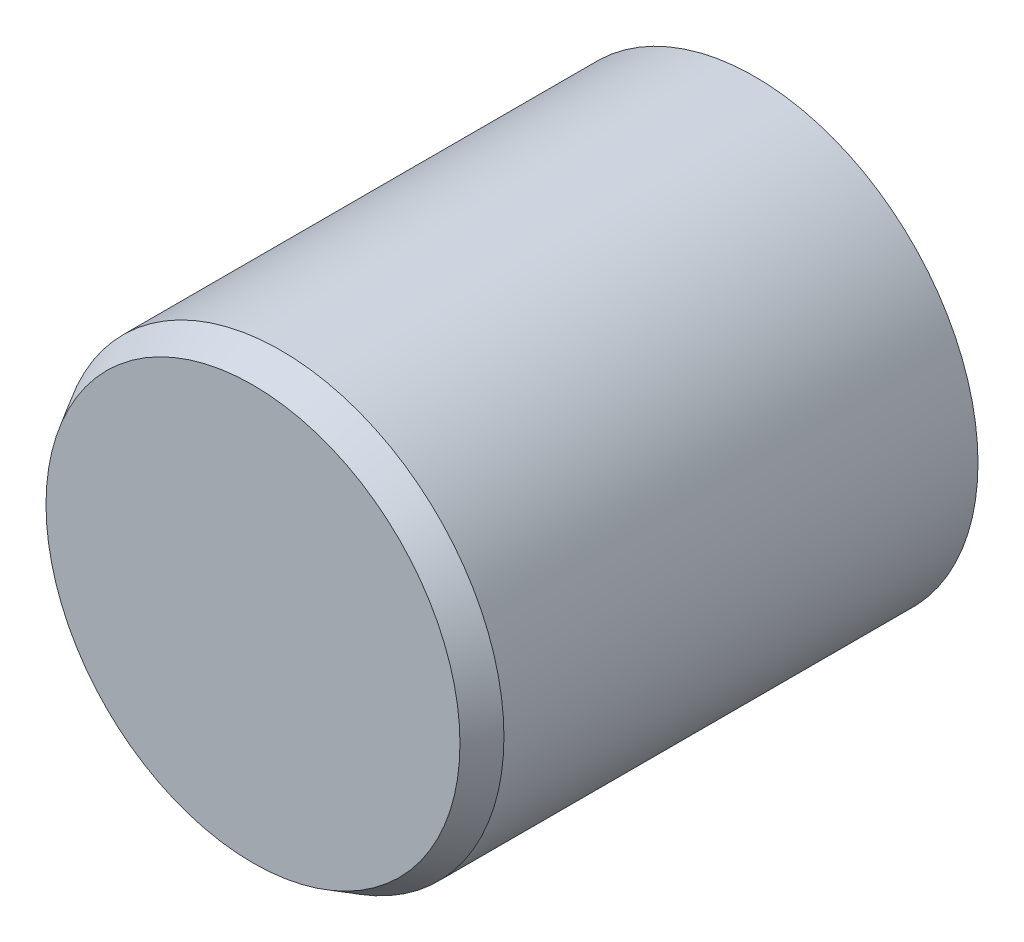
ISO-10303-21;
HEADER;
FILE_DESCRIPTION(('STEP AP214'),'2;1');
FILE_NAME('part.step','',(''),(''),'','','');
FILE_SCHEMA(('AUTOMOTIVE_DESIGN { 1 0 10303 214 1 1 1 1 }'));
ENDSEC;
DATA;
#1=APPLICATION_CONTEXT('core data for automotive mechanical design processes');
#2=APPLICATION_PROTOCOL_DEFINITION('international standard','automotive_design',2000,#1);
#3=PRODUCT_CONTEXT('',#1,'mechanical');
#4=PRODUCT('Part','Part','',(#3));
#5=PRODUCT_RELATED_PRODUCT_CATEGORY('part','',(#4));
#6=PRODUCT_DEFINITION_FORMATION('','',#4);
#7=PRODUCT_DEFINITION_CONTEXT('part definition',#1,'design');
#8=PRODUCT_DEFINITION('design','',#6,#7);
#9=PRODUCT_DEFINITION_SHAPE('','',#8);
#10=(LENGTH_UNIT() NAMED_UNIT(*) SI_UNIT(.MILLI.,.METRE.));
#11=(NAMED_UNIT(*) PLANE_ANGLE_UNIT() SI_UNIT($,.RADIAN.));
#12=(NAMED_UNIT(*) SI_UNIT($,.STERADIAN.) SOLID_ANGLE_UNIT());
#13=UNCERTAINTY_MEASURE_WITH_UNIT(LENGTH_MEASURE(1.E-05),#10,'distance_accuracy_value','');
#14=(GEOMETRIC_REPRESENTATION_CONTEXT(3) GLOBAL_UNCERTAINTY_ASSIGNED_CONTEXT((#13)) GLOBAL_UNIT_ASSIGNED_CONTEXT((#10,
#11,#12)) REPRESENTATION_CONTEXT('',''));
#15=CARTESIAN_POINT('',(0.,0.,0.));
#16=DIRECTION('',(0.,0.,1.));
#17=DIRECTION('',(1.,0.,0.));
#18=AXIS2_PLACEMENT_3D('',#15,#16,#17);
#19=CARTESIAN_POINT('',(0.,1.03333333333333,9.));
#20=DIRECTION('',(0.,0.,1.));
#21=DIRECTION('',(1.,0.,0.));
#22=AXIS2_PLACEMENT_3D('',#19,#20,#21);
#23=CYLINDRICAL_SURFACE('',#22,2.5);
#24=CARTESIAN_POINT('',(0.,1.03333333333333,6.));
#25=DIRECTION('',(0.,0.,1.));
#26=DIRECTION('',(1.,0.,0.));
#27=AXIS2_PLACEMENT_3D('',#24,#25,#26);
#28=CIRCLE('',#27,2.5);
#29=CARTESIAN_POINT('',(2.5,1.03333333333333,6.));
#30=VERTEX_POINT('',#29);
#31=EDGE_CURVE('E67',#30,#30,#28,.T.);
#32=ORIENTED_EDGE('',*,*,#31,.T.);
#33=EDGE_LOOP('',(#32));
#34=FACE_BOUND('',#33,.T.);
#35=CARTESIAN_POINT('',(0.,1.03333333333333,0.));
#36=DIRECTION('',(0.,0.,1.));
#37=DIRECTION('',(1.,0.,0.));
#38=AXIS2_PLACEMENT_3D('',#35,#36,#37);
#39=CIRCLE('',#38,2.5);
#40=CARTESIAN_POINT('',(2.5,1.03333333333333,0.));
#41=VERTEX_POINT('',#40);
#42=EDGE_CURVE('E60',#41,#41,#39,.T.);
#43=ORIENTED_EDGE('',*,*,#42,.F.);
#44=EDGE_LOOP('',(#43));
#45=FACE_BOUND('',#44,.T.);
#46=ADVANCED_FACE('F44',(#34,#45),#23,.F.);
#47=CARTESIAN_POINT('',(0.,-1.46666666666667,0.));
#48=DIRECTION('',(0.,0.,-1.));
#49=DIRECTION('',(-1.,0.,0.));
#50=AXIS2_PLACEMENT_3D('',#47,#48,#49);
#51=PLANE('',#50);
#52=ORIENTED_EDGE('',*,*,#42,.T.);
#53=EDGE_LOOP('',(#52));
#54=FACE_BOUND('',#53,.T.);
#55=CARTESIAN_POINT('',(0.,1.03333333333333,0.));
#56=DIRECTION('',(0.,0.,1.));
#57=DIRECTION('',(1.,0.,0.));
#58=AXIS2_PLACEMENT_3D('',#55,#56,#57);
#59=CIRCLE('',#58,4.);
#60=CARTESIAN_POINT('',(4.,1.03333333333333,0.));
#61=VERTEX_POINT('',#60);
#62=EDGE_CURVE('E64',#61,#61,#59,.T.);
#63=ORIENTED_EDGE('',*,*,#62,.F.);
#64=EDGE_LOOP('',(#63));
#65=FACE_BOUND('',#64,.T.);
#66=ADVANCED_FACE('F81',(#54,#65),#51,.T.);
#67=CARTESIAN_POINT('',(0.,1.03333333333333,9.));
#68=DIRECTION('',(0.,0.,1.));
#69=DIRECTION('',(1.,0.,0.));
#70=AXIS2_PLACEMENT_3D('',#67,#68,#69);
#71=CYLINDRICAL_SURFACE('',#70,4.);
#72=CARTESIAN_POINT('',(0.,1.03333333333333,8.5));
#73=DIRECTION('',(0.,0.,1.));
#74=DIRECTION('',(1.,0.,0.));
#75=AXIS2_PLACEMENT_3D('',#72,#73,#74);
#76=CIRCLE('',#75,4.);
#77=CARTESIAN_POINT('',(4.,1.03333333333333,8.5));
#78=VERTEX_POINT('',#77);
#79=EDGE_CURVE('E10',#78,#78,#76,.F.);
#80=ORIENTED_EDGE('',*,*,#79,.T.);
#81=EDGE_LOOP('',(#80));
#82=FACE_BOUND('',#81,.T.);
#83=ORIENTED_EDGE('',*,*,#62,.T.);
#84=EDGE_LOOP('',(#83));
#85=FACE_BOUND('',#84,.T.);
#86=ADVANCED_FACE('F85',(#82,#85),#71,.T.);
#87=CARTESIAN_POINT('',(0.,-2.96666666666667,9.));
#88=DIRECTION('',(0.,0.,1.));
#89=DIRECTION('',(1.,0.,0.));
#90=AXIS2_PLACEMENT_3D('',#87,#88,#89);
#91=PLANE('',#90);
#92=CARTESIAN_POINT('',(0.,1.03333333333333,9.));
#93=DIRECTION('',(0.,0.,1.));
#94=DIRECTION('',(1.,0.,0.));
#95=AXIS2_PLACEMENT_3D('',#92,#93,#94);
#96=CIRCLE('',#95,3.71132486540519);
#97=CARTESIAN_POINT('',(3.71132486540519,1.03333333333333,9.));
#98=VERTEX_POINT('',#97);
#99=EDGE_CURVE('E52',#98,#98,#96,.T.);
#100=ORIENTED_EDGE('',*,*,#99,.T.);
#101=EDGE_LOOP('',(#100));
#102=FACE_BOUND('',#101,.T.);
#103=ADVANCED_FACE('F74',(#102),#91,.T.);
#104=CARTESIAN_POINT('',(0.,1.03333333333333,6.));
#105=DIRECTION('',(0.,0.,-1.));
#106=DIRECTION('',(-1.,0.,0.));
#107=AXIS2_PLACEMENT_3D('',#104,#105,#106);
#108=PLANE('',#107);
#109=ORIENTED_EDGE('',*,*,#31,.F.);
#110=EDGE_LOOP('',(#109));
#111=FACE_BOUND('',#110,.T.);
#112=ADVANCED_FACE('F75',(#111),#108,.T.);
#113=CARTESIAN_POINT('',(0.,1.03333333333333,9.));
#114=DIRECTION('',(0.,0.,-1.));
#115=DIRECTION('',(-1.,0.,0.));
#116=AXIS2_PLACEMENT_3D('',#113,#114,#115);
#117=CONICAL_SURFACE('',#116,3.71132486540519,0.523598775598298);
#118=ORIENTED_EDGE('',*,*,#79,.F.);
#119=EDGE_LOOP('',(#118));
#120=FACE_BOUND('',#119,.T.);
#121=ORIENTED_EDGE('',*,*,#99,.F.);
#122=EDGE_LOOP('',(#121));
#123=FACE_BOUND('',#122,.T.);
#124=ADVANCED_FACE('F48',(#120,#123),#117,.T.);
#125=CLOSED_SHELL('',(#46,#66,#86,#103,#112,#124));
#126=MANIFOLD_SOLID_BREP('B2',#125);
#127=ADVANCED_BREP_SHAPE_REPRESENTATION('',(#18,#126),#14);
#128=SHAPE_DEFINITION_REPRESENTATION(#9,#127);
ENDSEC;
END-ISO-10303-21;
